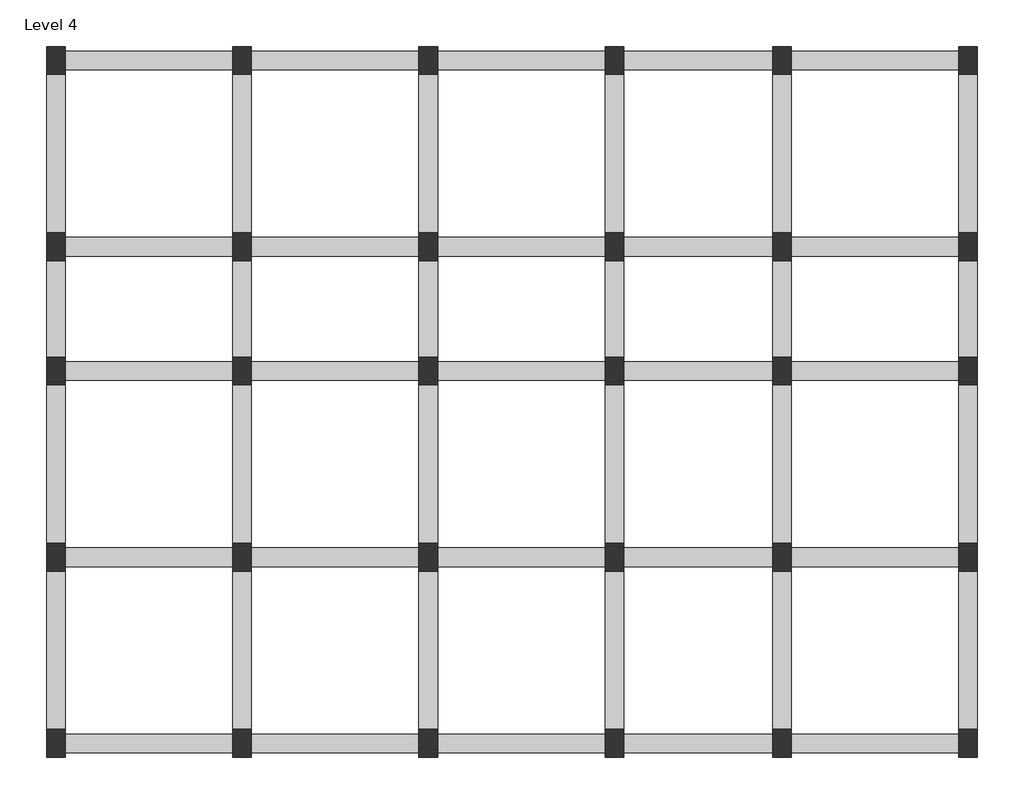
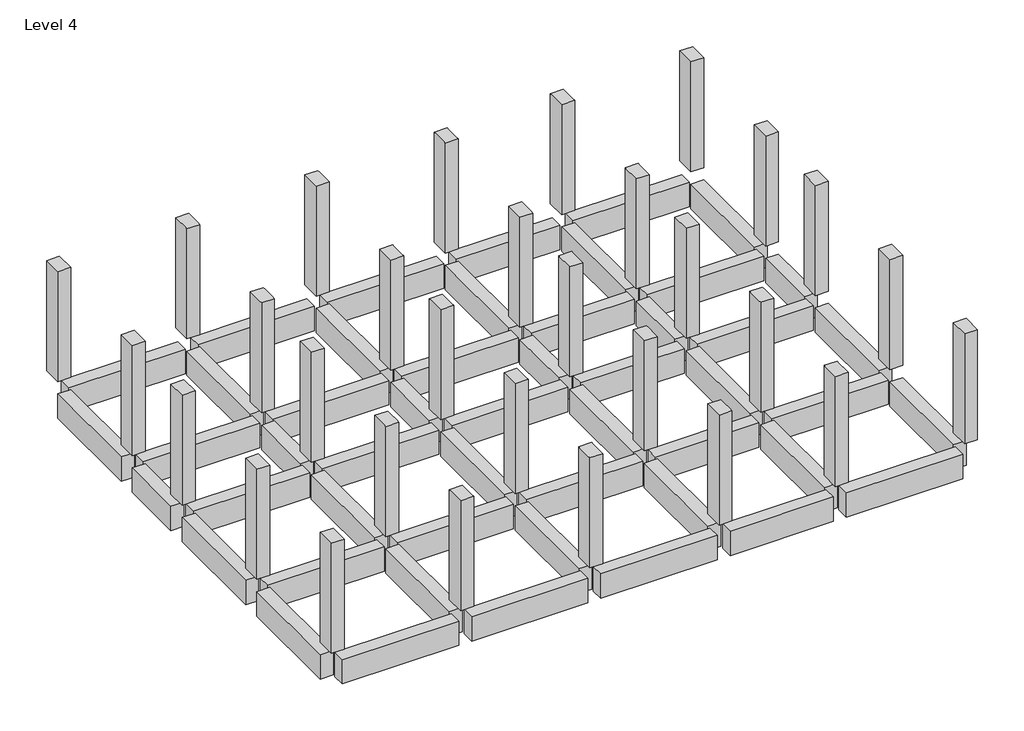
# One storey: 30 columns, 11 beams.
"""IFC4 building model written with IfcOpenShell, lengths in millimetres."""

from ifc_helpers import new_model, si_unit, frame, origin, place, context, project, spatial, polyline, outline, extrude, faceted_brep, element, save

model = new_model("IFC4")

# Units and contexts
model_context = context("Model", 3, world=origin())
ifc_project = project(units=[si_unit("LENGTHUNIT", "METRE", prefix="MILLI")], contexts=[model_context])

# Site, building, storey
site = spatial("IfcSite", under=ifc_project)
building = spatial("IfcBuilding", under=site)
storey = spatial("IfcBuildingStorey", under=building, Name="Level 4", Elevation=9144.0)

# Beams
placement = place(None, origin())
element("IfcBeam", 1, ObjectType="Concrete-Rectangular Beam : 12 x 24", at=placement, inside=storey, context=model_context, shape_type="SweptSolid", body=[
    extrude(outline(polyline([(2607.7603583, 7596.6647757), (2607.7603583, 7291.8647757), (-135.4396417, 7291.8647757), (-135.4396417, 7596.6647757), (2607.7603583, 7596.6647757)])), frame((0.0, 0.0, 8229.6), z_axis=(0.0, 0.0, 1.0), x_axis=(1.0, 0.0, 0.0)), (0.0, 0.0, 1.0), 609.6),
    extrude(outline(polyline([(-12022.6396417, 7291.8647757), (-12022.6396417, 7596.6647757), (-9279.4396417, 7596.6647757), (-9279.4396417, 7291.8647757), (-12022.6396417, 7291.8647757)])), frame((0.0, 0.0, 8229.6), z_axis=(0.0, 0.0, 1.0), x_axis=(1.0, 0.0, 0.0)), (0.0, 0.0, 1.0), 609.6),
    extrude(outline(polyline([(-8974.6396417, 7291.8647757), (-8974.6396417, 7596.6647757), (-6231.4396417, 7596.6647757), (-6231.4396417, 7291.8647757), (-8974.6396417, 7291.8647757)])), frame((0.0, 0.0, 8229.6), z_axis=(0.0, 0.0, 1.0), x_axis=(1.0, 0.0, 0.0)), (0.0, 0.0, 1.0), 609.6),
    extrude(outline(polyline([(-5926.6396417, 7291.8647757), (-5926.6396417, 7596.6647757), (-3183.4396417, 7596.6647757), (-3183.4396417, 7291.8647757), (-5926.6396417, 7291.8647757)])), frame((0.0, 0.0, 8229.6), z_axis=(0.0, 0.0, 1.0), x_axis=(1.0, 0.0, 0.0)), (0.0, 0.0, 1.0), 609.6),
    extrude(outline(polyline([(-2878.6396417, 7291.8647757), (-2878.6396417, 7596.6647757), (-440.2396417, 7596.6647757), (-440.2396417, 7291.8647757), (-2878.6396417, 7291.8647757)])), frame((0.0, 0.0, 8229.6), z_axis=(0.0, 0.0, 1.0), x_axis=(1.0, 0.0, 0.0)), (0.0, 0.0, 1.0), 609.6),
])
element("IfcBeam", 2, ObjectType="Concrete-Rectangular Beam : 12 x 24", at=placement, inside=storey, context=model_context, shape_type="SweptSolid", body=[
    extrude(outline(polyline([(2607.7603583, 10644.6647757), (2607.7603583, 10339.8647757), (-135.4396417, 10339.8647757), (-135.4396417, 10644.6647757), (2607.7603583, 10644.6647757)])), frame((0.0, 0.0, 8229.6), z_axis=(0.0, 0.0, 1.0), x_axis=(1.0, 0.0, 0.0)), (0.0, 0.0, 1.0), 609.6),
    extrude(outline(polyline([(-12022.6396417, 10339.8647757), (-12022.6396417, 10644.6647757), (-9279.4396417, 10644.6647757), (-9279.4396417, 10339.8647757), (-12022.6396417, 10339.8647757)])), frame((0.0, 0.0, 8229.6), z_axis=(0.0, 0.0, 1.0), x_axis=(1.0, 0.0, 0.0)), (0.0, 0.0, 1.0), 609.6),
    extrude(outline(polyline([(-8974.6396417, 10339.8647757), (-8974.6396417, 10644.6647757), (-6231.4396417, 10644.6647757), (-6231.4396417, 10339.8647757), (-8974.6396417, 10339.8647757)])), frame((0.0, 0.0, 8229.6), z_axis=(0.0, 0.0, 1.0), x_axis=(1.0, 0.0, 0.0)), (0.0, 0.0, 1.0), 609.6),
    extrude(outline(polyline([(-5926.6396417, 10339.8647757), (-5926.6396417, 10644.6647757), (-3183.4396417, 10644.6647757), (-3183.4396417, 10339.8647757), (-5926.6396417, 10339.8647757)])), frame((0.0, 0.0, 8229.6), z_axis=(0.0, 0.0, 1.0), x_axis=(1.0, 0.0, 0.0)), (0.0, 0.0, 1.0), 609.6),
    extrude(outline(polyline([(-2878.6396417, 10339.8647757), (-2878.6396417, 10644.6647757), (-440.2396417, 10644.6647757), (-440.2396417, 10339.8647757), (-2878.6396417, 10339.8647757)])), frame((0.0, 0.0, 8229.6), z_axis=(0.0, 0.0, 1.0), x_axis=(1.0, 0.0, 0.0)), (0.0, 0.0, 1.0), 609.6),
])
element("IfcBeam", 3, ObjectType="Concrete-Rectangular Beam : 12 x 24", at=placement, inside=storey, context=model_context, shape_type="SweptSolid", body=[
    extrude(outline(polyline([(2607.7603583, 13692.6647757), (2607.7603583, 13387.8647757), (-135.4396417, 13387.8647757), (-135.4396417, 13692.6647757), (2607.7603583, 13692.6647757)])), frame((0.0, 0.0, 8229.6), z_axis=(0.0, 0.0, 1.0), x_axis=(1.0, 0.0, 0.0)), (0.0, 0.0, 1.0), 609.6),
    extrude(outline(polyline([(-12022.6396417, 13387.8647757), (-12022.6396417, 13692.6647757), (-9279.4396417, 13692.6647757), (-9279.4396417, 13387.8647757), (-12022.6396417, 13387.8647757)])), frame((0.0, 0.0, 8229.6), z_axis=(0.0, 0.0, 1.0), x_axis=(1.0, 0.0, 0.0)), (0.0, 0.0, 1.0), 609.6),
    extrude(outline(polyline([(-8974.6396417, 13387.8647757), (-8974.6396417, 13692.6647757), (-6231.4396417, 13692.6647757), (-6231.4396417, 13387.8647757), (-8974.6396417, 13387.8647757)])), frame((0.0, 0.0, 8229.6), z_axis=(0.0, 0.0, 1.0), x_axis=(1.0, 0.0, 0.0)), (0.0, 0.0, 1.0), 609.6),
    extrude(outline(polyline([(-5926.6396417, 13387.8647757), (-5926.6396417, 13692.6647757), (-3183.4396417, 13692.6647757), (-3183.4396417, 13387.8647757), (-5926.6396417, 13387.8647757)])), frame((0.0, 0.0, 8229.6), z_axis=(0.0, 0.0, 1.0), x_axis=(1.0, 0.0, 0.0)), (0.0, 0.0, 1.0), 609.6),
    extrude(outline(polyline([(-2878.6396417, 13387.8647757), (-2878.6396417, 13692.6647757), (-440.2396417, 13692.6647757), (-440.2396417, 13387.8647757), (-2878.6396417, 13387.8647757)])), frame((0.0, 0.0, 8229.6), z_axis=(0.0, 0.0, 1.0), x_axis=(1.0, 0.0, 0.0)), (0.0, 0.0, 1.0), 609.6),
])
element("IfcBeam", 4, ObjectType="Concrete-Rectangular Beam : 12 x 24", at=placement, inside=storey, context=model_context, shape_type="SweptSolid", body=[
    extrude(outline(polyline([(2607.7603583, 15727.9119241), (2607.7603583, 15423.1119241), (-135.4396417, 15423.1119241), (-135.4396417, 15727.9119241), (2607.7603583, 15727.9119241)])), frame((0.0, 0.0, 8229.6), z_axis=(0.0, 0.0, 1.0), x_axis=(1.0, 0.0, 0.0)), (0.0, 0.0, 1.0), 609.6),
    extrude(outline(polyline([(-12022.6396417, 15423.1119241), (-12022.6396417, 15727.9119241), (-9279.4396417, 15727.9119241), (-9279.4396417, 15423.1119241), (-12022.6396417, 15423.1119241)])), frame((0.0, 0.0, 8229.6), z_axis=(0.0, 0.0, 1.0), x_axis=(1.0, 0.0, 0.0)), (0.0, 0.0, 1.0), 609.6),
    extrude(outline(polyline([(-8974.6396417, 15423.1119241), (-8974.6396417, 15727.9119241), (-6231.4396417, 15727.9119241), (-6231.4396417, 15423.1119241), (-8974.6396417, 15423.1119241)])), frame((0.0, 0.0, 8229.6), z_axis=(0.0, 0.0, 1.0), x_axis=(1.0, 0.0, 0.0)), (0.0, 0.0, 1.0), 609.6),
    extrude(outline(polyline([(-5926.6396417, 15423.1119241), (-5926.6396417, 15727.9119241), (-3183.4396417, 15727.9119241), (-3183.4396417, 15423.1119241), (-5926.6396417, 15423.1119241)])), frame((0.0, 0.0, 8229.6), z_axis=(0.0, 0.0, 1.0), x_axis=(1.0, 0.0, 0.0)), (0.0, 0.0, 1.0), 609.6),
    extrude(outline(polyline([(-2878.6396417, 15423.1119241), (-2878.6396417, 15727.9119241), (-440.2396417, 15727.9119241), (-440.2396417, 15423.1119241), (-2878.6396417, 15423.1119241)])), frame((0.0, 0.0, 8229.6), z_axis=(0.0, 0.0, 1.0), x_axis=(1.0, 0.0, 0.0)), (0.0, 0.0, 1.0), 609.6),
])
element("IfcBeam", 5, ObjectType="Concrete-Rectangular Beam : 12 x 24", at=placement, inside=storey, context=model_context, shape_type="SweptSolid", body=[
    extrude(outline(polyline([(2607.7603583, 18775.9119241), (2607.7603583, 18471.1119241), (-135.4396417, 18471.1119241), (-135.4396417, 18775.9119241), (2607.7603583, 18775.9119241)])), frame((0.0, 0.0, 8229.6), z_axis=(0.0, 0.0, 1.0), x_axis=(1.0, 0.0, 0.0)), (0.0, 0.0, 1.0), 609.6),
    extrude(outline(polyline([(-12022.6396417, 18471.1119241), (-12022.6396417, 18775.9119241), (-9279.4396417, 18775.9119241), (-9279.4396417, 18471.1119241), (-12022.6396417, 18471.1119241)])), frame((0.0, 0.0, 8229.6), z_axis=(0.0, 0.0, 1.0), x_axis=(1.0, 0.0, 0.0)), (0.0, 0.0, 1.0), 609.6),
    extrude(outline(polyline([(-8974.6396417, 18471.1119241), (-8974.6396417, 18775.9119241), (-6231.4396417, 18775.9119241), (-6231.4396417, 18471.1119241), (-8974.6396417, 18471.1119241)])), frame((0.0, 0.0, 8229.6), z_axis=(0.0, 0.0, 1.0), x_axis=(1.0, 0.0, 0.0)), (0.0, 0.0, 1.0), 609.6),
    extrude(outline(polyline([(-5926.6396417, 18471.1119241), (-5926.6396417, 18775.9119241), (-3183.4396417, 18775.9119241), (-3183.4396417, 18471.1119241), (-5926.6396417, 18471.1119241)])), frame((0.0, 0.0, 8229.6), z_axis=(0.0, 0.0, 1.0), x_axis=(1.0, 0.0, 0.0)), (0.0, 0.0, 1.0), 609.6),
    extrude(outline(polyline([(-2878.6396417, 18471.1119241), (-2878.6396417, 18775.9119241), (-440.2396417, 18775.9119241), (-440.2396417, 18471.1119241), (-2878.6396417, 18471.1119241)])), frame((0.0, 0.0, 8229.6), z_axis=(0.0, 0.0, 1.0), x_axis=(1.0, 0.0, 0.0)), (0.0, 0.0, 1.0), 609.6),
])
element("IfcBeam", 6, ObjectType="Concrete-Rectangular Beam : 12 x 24", at=placement, inside=storey, context=model_context, shape_type="SweptSolid", body=[
    extrude(outline(polyline([(-12022.6396417, 7672.8647757), (-12327.4396417, 7672.8647757), (-12327.4396417, 10263.6647757), (-12022.6396417, 10263.6647757), (-12022.6396417, 7672.8647757)])), frame((0.0, 0.0, 8229.6), z_axis=(0.0, 0.0, 1.0), x_axis=(1.0, 0.0, 0.0)), (0.0, 0.0, 1.0), 609.6),
    extrude(outline(polyline([(-12327.4396417, 18394.9119241), (-12022.6396417, 18394.9119241), (-12022.6396417, 15804.1119241), (-12327.4396417, 15804.1119241), (-12327.4396417, 18394.9119241)])), frame((0.0, 0.0, 8229.6), z_axis=(0.0, 0.0, 1.0), x_axis=(1.0, 0.0, 0.0)), (0.0, 0.0, 1.0), 609.6),
    extrude(outline(polyline([(-12022.6396417, 10720.8647757), (-12327.4396417, 10720.8647757), (-12327.4396417, 13311.6647757), (-12022.6396417, 13311.6647757), (-12022.6396417, 10720.8647757)])), frame((0.0, 0.0, 8229.6), z_axis=(0.0, 0.0, 1.0), x_axis=(1.0, 0.0, 0.0)), (0.0, 0.0, 1.0), 609.6),
    extrude(outline(polyline([(-12022.6396417, 13768.8647757), (-12327.4396417, 13768.8647757), (-12327.4396417, 15346.9119241), (-12022.6396417, 15346.9119241), (-12022.6396417, 13768.8647757)])), frame((0.0, 0.0, 8229.6), z_axis=(0.0, 0.0, 1.0), x_axis=(1.0, 0.0, 0.0)), (0.0, 0.0, 1.0), 609.6),
])
element("IfcBeam", 7, ObjectType="Concrete-Rectangular Beam : 12 x 24", at=placement, inside=storey, context=model_context, shape_type="SweptSolid", body=[
    extrude(outline(polyline([(-8974.6396417, 7672.8647757), (-9279.4396417, 7672.8647757), (-9279.4396417, 10263.6647757), (-8974.6396417, 10263.6647757), (-8974.6396417, 7672.8647757)])), frame((0.0, 0.0, 8229.6), z_axis=(0.0, 0.0, 1.0), x_axis=(1.0, 0.0, 0.0)), (0.0, 0.0, 1.0), 609.6),
    extrude(outline(polyline([(-9279.4396417, 18394.9119241), (-8974.6396417, 18394.9119241), (-8974.6396417, 15804.1119241), (-9279.4396417, 15804.1119241), (-9279.4396417, 18394.9119241)])), frame((0.0, 0.0, 8229.6), z_axis=(0.0, 0.0, 1.0), x_axis=(1.0, 0.0, 0.0)), (0.0, 0.0, 1.0), 609.6),
    extrude(outline(polyline([(-8974.6396417, 10720.8647757), (-9279.4396417, 10720.8647757), (-9279.4396417, 13311.6647757), (-8974.6396417, 13311.6647757), (-8974.6396417, 10720.8647757)])), frame((0.0, 0.0, 8229.6), z_axis=(0.0, 0.0, 1.0), x_axis=(1.0, 0.0, 0.0)), (0.0, 0.0, 1.0), 609.6),
    extrude(outline(polyline([(-8974.6396417, 13768.8647757), (-9279.4396417, 13768.8647757), (-9279.4396417, 15346.9119241), (-8974.6396417, 15346.9119241), (-8974.6396417, 13768.8647757)])), frame((0.0, 0.0, 8229.6), z_axis=(0.0, 0.0, 1.0), x_axis=(1.0, 0.0, 0.0)), (0.0, 0.0, 1.0), 609.6),
])
element("IfcBeam", 8, ObjectType="Concrete-Rectangular Beam : 12 x 24", at=placement, inside=storey, context=model_context, shape_type="SweptSolid", body=[
    extrude(outline(polyline([(-5926.6396417, 7672.8647757), (-6231.4396417, 7672.8647757), (-6231.4396417, 10263.6647757), (-5926.6396417, 10263.6647757), (-5926.6396417, 7672.8647757)])), frame((0.0, 0.0, 8229.6), z_axis=(0.0, 0.0, 1.0), x_axis=(1.0, 0.0, 0.0)), (0.0, 0.0, 1.0), 609.6),
    extrude(outline(polyline([(-6231.4396417, 18394.9119241), (-5926.6396417, 18394.9119241), (-5926.6396417, 15804.1119241), (-6231.4396417, 15804.1119241), (-6231.4396417, 18394.9119241)])), frame((0.0, 0.0, 8229.6), z_axis=(0.0, 0.0, 1.0), x_axis=(1.0, 0.0, 0.0)), (0.0, 0.0, 1.0), 609.6),
    extrude(outline(polyline([(-5926.6396417, 10720.8647757), (-6231.4396417, 10720.8647757), (-6231.4396417, 13311.6647757), (-5926.6396417, 13311.6647757), (-5926.6396417, 10720.8647757)])), frame((0.0, 0.0, 8229.6), z_axis=(0.0, 0.0, 1.0), x_axis=(1.0, 0.0, 0.0)), (0.0, 0.0, 1.0), 609.6),
    extrude(outline(polyline([(-5926.6396417, 13768.8647757), (-6231.4396417, 13768.8647757), (-6231.4396417, 15346.9119241), (-5926.6396417, 15346.9119241), (-5926.6396417, 13768.8647757)])), frame((0.0, 0.0, 8229.6), z_axis=(0.0, 0.0, 1.0), x_axis=(1.0, 0.0, 0.0)), (0.0, 0.0, 1.0), 609.6),
])
element("IfcBeam", 9, ObjectType="Concrete-Rectangular Beam : 12 x 24", at=placement, inside=storey, context=model_context, shape_type="SweptSolid", body=[
    extrude(outline(polyline([(-2878.6396417, 7672.8647757), (-3183.4396417, 7672.8647757), (-3183.4396417, 10263.6647757), (-2878.6396417, 10263.6647757), (-2878.6396417, 7672.8647757)])), frame((0.0, 0.0, 8229.6), z_axis=(0.0, 0.0, 1.0), x_axis=(1.0, 0.0, 0.0)), (0.0, 0.0, 1.0), 609.6),
    extrude(outline(polyline([(-3183.4396417, 18394.9119241), (-2878.6396417, 18394.9119241), (-2878.6396417, 15804.1119241), (-3183.4396417, 15804.1119241), (-3183.4396417, 18394.9119241)])), frame((0.0, 0.0, 8229.6), z_axis=(0.0, 0.0, 1.0), x_axis=(1.0, 0.0, 0.0)), (0.0, 0.0, 1.0), 609.6),
    extrude(outline(polyline([(-2878.6396417, 10720.8647757), (-3183.4396417, 10720.8647757), (-3183.4396417, 13311.6647757), (-2878.6396417, 13311.6647757), (-2878.6396417, 10720.8647757)])), frame((0.0, 0.0, 8229.6), z_axis=(0.0, 0.0, 1.0), x_axis=(1.0, 0.0, 0.0)), (0.0, 0.0, 1.0), 609.6),
    extrude(outline(polyline([(-2878.6396417, 13768.8647757), (-3183.4396417, 13768.8647757), (-3183.4396417, 15346.9119241), (-2878.6396417, 15346.9119241), (-2878.6396417, 13768.8647757)])), frame((0.0, 0.0, 8229.6), z_axis=(0.0, 0.0, 1.0), x_axis=(1.0, 0.0, 0.0)), (0.0, 0.0, 1.0), 609.6),
])
element("IfcBeam", 10, ObjectType="Concrete-Rectangular Beam : 12 x 24", at=placement, inside=storey, context=model_context, shape_type="SweptSolid", body=[
    extrude(outline(polyline([(-135.4396417, 7672.8647757), (-440.2396417, 7672.8647757), (-440.2396417, 10263.6647757), (-135.4396417, 10263.6647757), (-135.4396417, 7672.8647757)])), frame((0.0, 0.0, 8229.6), z_axis=(0.0, 0.0, 1.0), x_axis=(1.0, 0.0, 0.0)), (0.0, 0.0, 1.0), 609.6),
    extrude(outline(polyline([(-440.2396417, 18394.9119241), (-135.4396417, 18394.9119241), (-135.4396417, 15804.1119241), (-440.2396417, 15804.1119241), (-440.2396417, 18394.9119241)])), frame((0.0, 0.0, 8229.6), z_axis=(0.0, 0.0, 1.0), x_axis=(1.0, 0.0, 0.0)), (0.0, 0.0, 1.0), 609.6),
    extrude(outline(polyline([(-135.4396417, 10720.8647757), (-440.2396417, 10720.8647757), (-440.2396417, 13311.6647757), (-135.4396417, 13311.6647757), (-135.4396417, 10720.8647757)])), frame((0.0, 0.0, 8229.6), z_axis=(0.0, 0.0, 1.0), x_axis=(1.0, 0.0, 0.0)), (0.0, 0.0, 1.0), 609.6),
    extrude(outline(polyline([(-135.4396417, 13768.8647757), (-440.2396417, 13768.8647757), (-440.2396417, 15346.9119241), (-135.4396417, 15346.9119241), (-135.4396417, 13768.8647757)])), frame((0.0, 0.0, 8229.6), z_axis=(0.0, 0.0, 1.0), x_axis=(1.0, 0.0, 0.0)), (0.0, 0.0, 1.0), 609.6),
])
element("IfcBeam", 11, ObjectType="Concrete-Rectangular Beam : 12 x 24", at=placement, inside=storey, context=model_context, shape_type="SweptSolid", body=[
    extrude(outline(polyline([(2912.5603583, 7672.8647757), (2607.7603583, 7672.8647757), (2607.7603583, 10263.6647757), (2912.5603583, 10263.6647757), (2912.5603583, 7672.8647757)])), frame((0.0, 0.0, 8229.6), z_axis=(0.0, 0.0, 1.0), x_axis=(1.0, 0.0, 0.0)), (0.0, 0.0, 1.0), 609.6),
    extrude(outline(polyline([(2607.7603583, 18394.9119241), (2912.5603583, 18394.9119241), (2912.5603583, 15804.1119241), (2607.7603583, 15804.1119241), (2607.7603583, 18394.9119241)])), frame((0.0, 0.0, 8229.6), z_axis=(0.0, 0.0, 1.0), x_axis=(1.0, 0.0, 0.0)), (0.0, 0.0, 1.0), 609.6),
    extrude(outline(polyline([(2912.5603583, 10720.8647757), (2607.7603583, 10720.8647757), (2607.7603583, 13311.6647757), (2912.5603583, 13311.6647757), (2912.5603583, 10720.8647757)])), frame((0.0, 0.0, 8229.6), z_axis=(0.0, 0.0, 1.0), x_axis=(1.0, 0.0, 0.0)), (0.0, 0.0, 1.0), 609.6),
    extrude(outline(polyline([(2912.5603583, 13768.8647757), (2607.7603583, 13768.8647757), (2607.7603583, 15346.9119241), (2912.5603583, 15346.9119241), (2912.5603583, 13768.8647757)])), frame((0.0, 0.0, 8229.6), z_axis=(0.0, 0.0, 1.0), x_axis=(1.0, 0.0, 0.0)), (0.0, 0.0, 1.0), 609.6),
])

# Columns
element("IfcColumn", 12, ObjectType="Concrete-Rectangular-Column : c1", at=placement, inside=storey, context=model_context, shape_type="SweptSolid", body=[
    extrude(outline(polyline([(-12327.4396417, 7215.6647757), (-12327.4396417, 7672.8647757), (-12022.6396417, 7672.8647757), (-12022.6396417, 7215.6647757), (-12327.4396417, 7215.6647757)])), frame((0.0, 0.0, 9144.0), z_axis=(0.0, 0.0, 1.0), x_axis=(1.0, 0.0, 0.0)), (0.0, 0.0, 1.0), 2743.2),
])
element("IfcColumn", 13, ObjectType="Concrete-Rectangular-Column : c1", at=placement, inside=storey, context=model_context, shape_type="Brep", body=[
    faceted_brep([(-9279.4396417, 7215.6647757, 9144.0), (-9279.4396417, 7672.8647757, 9144.0), (-8974.6396417, 7672.8647757, 9144.0), (-8974.6396417, 7215.6647757, 9144.0), (-9279.4396417, 7215.6647757, 11887.2), (-9279.4396417, 7291.8647757, 11887.2), (-9279.4396417, 7596.6647757, 11887.2), (-9279.4396417, 7672.8647757, 11887.2), (-8974.6396417, 7672.8647757, 11887.2), (-8974.6396417, 7596.6647757, 11887.2), (-8974.6396417, 7291.8647757, 11887.2), (-8974.6396417, 7215.6647757, 11887.2)], [[[0, 1, 2, 3]], [[4, 5, 6, 7, 1, 0]], [[7, 8, 2, 1]], [[8, 9, 10, 11, 3, 2]], [[11, 4, 0, 3]], [[4, 11, 10, 9, 8, 7, 6, 5]]]),
])
element("IfcColumn", 14, ObjectType="Concrete-Rectangular-Column : c1", at=placement, inside=storey, context=model_context, shape_type="Brep", body=[
    faceted_brep([(-6231.4396417, 7215.6647757, 9144.0), (-6231.4396417, 7672.8647757, 9144.0), (-5926.6396417, 7672.8647757, 9144.0), (-5926.6396417, 7215.6647757, 9144.0), (-6231.4396417, 7215.6647757, 11887.2), (-6231.4396417, 7291.8647757, 11887.2), (-6231.4396417, 7596.6647757, 11887.2), (-6231.4396417, 7672.8647757, 11887.2), (-5926.6396417, 7672.8647757, 11887.2), (-5926.6396417, 7596.6647757, 11887.2), (-5926.6396417, 7291.8647757, 11887.2), (-5926.6396417, 7215.6647757, 11887.2)], [[[0, 1, 2, 3]], [[4, 5, 6, 7, 1, 0]], [[7, 8, 2, 1]], [[8, 9, 10, 11, 3, 2]], [[11, 4, 0, 3]], [[4, 11, 10, 9, 8, 7, 6, 5]]]),
])
element("IfcColumn", 15, ObjectType="Concrete-Rectangular-Column : c1", at=placement, inside=storey, context=model_context, shape_type="Brep", body=[
    faceted_brep([(-3183.4396417, 7215.6647757, 9144.0), (-3183.4396417, 7672.8647757, 9144.0), (-2878.6396417, 7672.8647757, 9144.0), (-2878.6396417, 7215.6647757, 9144.0), (-3183.4396417, 7215.6647757, 11887.2), (-3183.4396417, 7291.8647757, 11887.2), (-3183.4396417, 7596.6647757, 11887.2), (-3183.4396417, 7672.8647757, 11887.2), (-2878.6396417, 7672.8647757, 11887.2), (-2878.6396417, 7596.6647757, 11887.2), (-2878.6396417, 7291.8647757, 11887.2), (-2878.6396417, 7215.6647757, 11887.2)], [[[0, 1, 2, 3]], [[4, 5, 6, 7, 1, 0]], [[7, 8, 2, 1]], [[8, 9, 10, 11, 3, 2]], [[11, 4, 0, 3]], [[4, 11, 10, 9, 8, 7, 6, 5]]]),
])
element("IfcColumn", 16, ObjectType="Concrete-Rectangular-Column : c1", at=placement, inside=storey, context=model_context, shape_type="Brep", body=[
    faceted_brep([(-440.2396417, 7215.6647757, 9144.0), (-440.2396417, 7672.8647757, 9144.0), (-135.4396417, 7672.8647757, 9144.0), (-135.4396417, 7215.6647757, 9144.0), (-440.2396417, 7215.6647757, 11887.2), (-440.2396417, 7291.8647757, 11887.2), (-440.2396417, 7596.6647757, 11887.2), (-440.2396417, 7672.8647757, 11887.2), (-135.4396417, 7672.8647757, 11887.2), (-135.4396417, 7596.6647757, 11887.2), (-135.4396417, 7291.8647757, 11887.2), (-135.4396417, 7215.6647757, 11887.2)], [[[0, 1, 2, 3]], [[4, 5, 6, 7, 1, 0]], [[7, 8, 2, 1]], [[8, 9, 10, 11, 3, 2]], [[11, 4, 0, 3]], [[4, 11, 10, 9, 8, 7, 6, 5]]]),
])
element("IfcColumn", 17, ObjectType="Concrete-Rectangular-Column : c1", at=placement, inside=storey, context=model_context, shape_type="SweptSolid", body=[
    extrude(outline(polyline([(2607.7603583, 7215.6647757), (2607.7603583, 7672.8647757), (2912.5603583, 7672.8647757), (2912.5603583, 7215.6647757), (2607.7603583, 7215.6647757)])), frame((0.0, 0.0, 9144.0), z_axis=(0.0, 0.0, 1.0), x_axis=(1.0, 0.0, 0.0)), (0.0, 0.0, 1.0), 2743.2),
])
element("IfcColumn", 18, ObjectType="Concrete-Rectangular-Column : c1", at=placement, inside=storey, context=model_context, shape_type="Brep", body=[
    faceted_brep([(-12327.4396417, 10263.6647757, 9144.0), (-12327.4396417, 10720.8647757, 9144.0), (-12022.6396417, 10720.8647757, 9144.0), (-12022.6396417, 10263.6647757, 9144.0), (-12327.4396417, 10263.6647757, 11887.2), (-12327.4396417, 10720.8647757, 11887.2), (-12327.4396417, 10720.8647757, 11277.6), (-12327.4396417, 10263.6647757, 11277.6), (-12022.6396417, 10720.8647757, 11887.2), (-12022.6396417, 10720.8647757, 11277.6), (-12022.6396417, 10263.6647757, 11887.2), (-12022.6396417, 10263.6647757, 11277.6)], [[[0, 1, 2, 3]], [[4, 5, 6, 1, 0, 7]], [[5, 8, 9, 2, 1, 6]], [[8, 10, 11, 3, 2, 9]], [[10, 4, 7, 0, 3, 11]], [[4, 10, 8, 5]]]),
])
element("IfcColumn", 19, ObjectType="Concrete-Rectangular-Column : c1", at=placement, inside=storey, context=model_context, shape_type="Brep", body=[
    faceted_brep([(-9279.4396417, 10263.6647757, 9144.0), (-9279.4396417, 10720.8647757, 9144.0), (-8974.6396417, 10720.8647757, 9144.0), (-8974.6396417, 10263.6647757, 9144.0), (-9279.4396417, 10263.6647757, 11887.2), (-9279.4396417, 10339.8647757, 11887.2), (-9279.4396417, 10644.6647757, 11887.2), (-9279.4396417, 10720.8647757, 11887.2), (-9279.4396417, 10720.8647757, 11277.6), (-9279.4396417, 10263.6647757, 11277.6), (-8974.6396417, 10720.8647757, 11887.2), (-8974.6396417, 10720.8647757, 11277.6), (-8974.6396417, 10644.6647757, 11887.2), (-8974.6396417, 10339.8647757, 11887.2), (-8974.6396417, 10263.6647757, 11887.2), (-8974.6396417, 10263.6647757, 11277.6)], [[[0, 1, 2, 3]], [[4, 5, 6, 7, 8, 1, 0, 9]], [[7, 10, 11, 2, 1, 8]], [[10, 12, 13, 14, 15, 3, 2, 11]], [[14, 4, 9, 0, 3, 15]], [[4, 14, 13, 12, 10, 7, 6, 5]]]),
])
element("IfcColumn", 20, ObjectType="Concrete-Rectangular-Column : c1", at=placement, inside=storey, context=model_context, shape_type="Brep", body=[
    faceted_brep([(-6231.4396417, 10263.6647757, 9144.0), (-6231.4396417, 10720.8647757, 9144.0), (-5926.6396417, 10720.8647757, 9144.0), (-5926.6396417, 10263.6647757, 9144.0), (-6231.4396417, 10263.6647757, 11887.2), (-6231.4396417, 10339.8647757, 11887.2), (-6231.4396417, 10644.6647757, 11887.2), (-6231.4396417, 10720.8647757, 11887.2), (-6231.4396417, 10720.8647757, 11277.6), (-6231.4396417, 10263.6647757, 11277.6), (-5926.6396417, 10720.8647757, 11887.2), (-5926.6396417, 10720.8647757, 11277.6), (-5926.6396417, 10644.6647757, 11887.2), (-5926.6396417, 10339.8647757, 11887.2), (-5926.6396417, 10263.6647757, 11887.2), (-5926.6396417, 10263.6647757, 11277.6)], [[[0, 1, 2, 3]], [[4, 5, 6, 7, 8, 1, 0, 9]], [[7, 10, 11, 2, 1, 8]], [[10, 12, 13, 14, 15, 3, 2, 11]], [[14, 4, 9, 0, 3, 15]], [[4, 14, 13, 12, 10, 7, 6, 5]]]),
])
element("IfcColumn", 21, ObjectType="Concrete-Rectangular-Column : c1", at=placement, inside=storey, context=model_context, shape_type="Brep", body=[
    faceted_brep([(-3183.4396417, 10263.6647757, 9144.0), (-3183.4396417, 10720.8647757, 9144.0), (-2878.6396417, 10720.8647757, 9144.0), (-2878.6396417, 10263.6647757, 9144.0), (-3183.4396417, 10263.6647757, 11887.2), (-3183.4396417, 10339.8647757, 11887.2), (-3183.4396417, 10644.6647757, 11887.2), (-3183.4396417, 10720.8647757, 11887.2), (-3183.4396417, 10720.8647757, 11277.6), (-3183.4396417, 10263.6647757, 11277.6), (-2878.6396417, 10720.8647757, 11887.2), (-2878.6396417, 10720.8647757, 11277.6), (-2878.6396417, 10644.6647757, 11887.2), (-2878.6396417, 10339.8647757, 11887.2), (-2878.6396417, 10263.6647757, 11887.2), (-2878.6396417, 10263.6647757, 11277.6)], [[[0, 1, 2, 3]], [[4, 5, 6, 7, 8, 1, 0, 9]], [[7, 10, 11, 2, 1, 8]], [[10, 12, 13, 14, 15, 3, 2, 11]], [[14, 4, 9, 0, 3, 15]], [[4, 14, 13, 12, 10, 7, 6, 5]]]),
])
element("IfcColumn", 22, ObjectType="Concrete-Rectangular-Column : c1", at=placement, inside=storey, context=model_context, shape_type="Brep", body=[
    faceted_brep([(-440.2396417, 10263.6647757, 9144.0), (-440.2396417, 10720.8647757, 9144.0), (-135.4396417, 10720.8647757, 9144.0), (-135.4396417, 10263.6647757, 9144.0), (-440.2396417, 10263.6647757, 11887.2), (-440.2396417, 10339.8647757, 11887.2), (-440.2396417, 10644.6647757, 11887.2), (-440.2396417, 10720.8647757, 11887.2), (-440.2396417, 10720.8647757, 11277.6), (-440.2396417, 10263.6647757, 11277.6), (-135.4396417, 10720.8647757, 11887.2), (-135.4396417, 10720.8647757, 11277.6), (-135.4396417, 10644.6647757, 11887.2), (-135.4396417, 10339.8647757, 11887.2), (-135.4396417, 10263.6647757, 11887.2), (-135.4396417, 10263.6647757, 11277.6)], [[[0, 1, 2, 3]], [[4, 5, 6, 7, 8, 1, 0, 9]], [[7, 10, 11, 2, 1, 8]], [[10, 12, 13, 14, 15, 3, 2, 11]], [[14, 4, 9, 0, 3, 15]], [[4, 14, 13, 12, 10, 7, 6, 5]]]),
])
element("IfcColumn", 23, ObjectType="Concrete-Rectangular-Column : c1", at=placement, inside=storey, context=model_context, shape_type="Brep", body=[
    faceted_brep([(2607.7603583, 10263.6647757, 9144.0), (2607.7603583, 10720.8647757, 9144.0), (2912.5603583, 10720.8647757, 9144.0), (2912.5603583, 10263.6647757, 9144.0), (2607.7603583, 10263.6647757, 11887.2), (2607.7603583, 10720.8647757, 11887.2), (2607.7603583, 10720.8647757, 11277.6), (2607.7603583, 10263.6647757, 11277.6), (2912.5603583, 10720.8647757, 11887.2), (2912.5603583, 10720.8647757, 11277.6), (2912.5603583, 10263.6647757, 11887.2), (2912.5603583, 10263.6647757, 11277.6)], [[[0, 1, 2, 3]], [[4, 5, 6, 1, 0, 7]], [[5, 8, 9, 2, 1, 6]], [[8, 10, 11, 3, 2, 9]], [[10, 4, 7, 0, 3, 11]], [[4, 10, 8, 5]]]),
])
element("IfcColumn", 24, ObjectType="Concrete-Rectangular-Column : c1", at=placement, inside=storey, context=model_context, shape_type="Brep", body=[
    faceted_brep([(-12327.4396417, 13311.6647757, 9144.0), (-12327.4396417, 13768.8647757, 9144.0), (-12022.6396417, 13768.8647757, 9144.0), (-12022.6396417, 13311.6647757, 9144.0), (-12327.4396417, 13311.6647757, 11887.2), (-12327.4396417, 13768.8647757, 11887.2), (-12327.4396417, 13768.8647757, 11277.6), (-12327.4396417, 13311.6647757, 11277.6), (-12022.6396417, 13768.8647757, 11887.2), (-12022.6396417, 13768.8647757, 11277.6), (-12022.6396417, 13311.6647757, 11887.2), (-12022.6396417, 13311.6647757, 11277.6)], [[[0, 1, 2, 3]], [[4, 5, 6, 1, 0, 7]], [[5, 8, 9, 2, 1, 6]], [[8, 10, 11, 3, 2, 9]], [[10, 4, 7, 0, 3, 11]], [[4, 10, 8, 5]]]),
])
element("IfcColumn", 25, ObjectType="Concrete-Rectangular-Column : c1", at=placement, inside=storey, context=model_context, shape_type="Brep", body=[
    faceted_brep([(-9279.4396417, 13311.6647757, 9144.0), (-9279.4396417, 13768.8647757, 9144.0), (-8974.6396417, 13768.8647757, 9144.0), (-8974.6396417, 13311.6647757, 9144.0), (-9279.4396417, 13311.6647757, 11887.2), (-9279.4396417, 13387.8647757, 11887.2), (-9279.4396417, 13692.6647757, 11887.2), (-9279.4396417, 13768.8647757, 11887.2), (-9279.4396417, 13768.8647757, 11277.6), (-9279.4396417, 13311.6647757, 11277.6), (-8974.6396417, 13768.8647757, 11887.2), (-8974.6396417, 13768.8647757, 11277.6), (-8974.6396417, 13692.6647757, 11887.2), (-8974.6396417, 13387.8647757, 11887.2), (-8974.6396417, 13311.6647757, 11887.2), (-8974.6396417, 13311.6647757, 11277.6)], [[[0, 1, 2, 3]], [[4, 5, 6, 7, 8, 1, 0, 9]], [[7, 10, 11, 2, 1, 8]], [[10, 12, 13, 14, 15, 3, 2, 11]], [[14, 4, 9, 0, 3, 15]], [[4, 14, 13, 12, 10, 7, 6, 5]]]),
])
element("IfcColumn", 26, ObjectType="Concrete-Rectangular-Column : c1", at=placement, inside=storey, context=model_context, shape_type="Brep", body=[
    faceted_brep([(-6231.4396417, 13311.6647757, 9144.0), (-6231.4396417, 13768.8647757, 9144.0), (-5926.6396417, 13768.8647757, 9144.0), (-5926.6396417, 13311.6647757, 9144.0), (-6231.4396417, 13311.6647757, 11887.2), (-6231.4396417, 13387.8647757, 11887.2), (-6231.4396417, 13692.6647757, 11887.2), (-6231.4396417, 13768.8647757, 11887.2), (-6231.4396417, 13768.8647757, 11277.6), (-6231.4396417, 13311.6647757, 11277.6), (-5926.6396417, 13768.8647757, 11887.2), (-5926.6396417, 13768.8647757, 11277.6), (-5926.6396417, 13692.6647757, 11887.2), (-5926.6396417, 13387.8647757, 11887.2), (-5926.6396417, 13311.6647757, 11887.2), (-5926.6396417, 13311.6647757, 11277.6)], [[[0, 1, 2, 3]], [[4, 5, 6, 7, 8, 1, 0, 9]], [[7, 10, 11, 2, 1, 8]], [[10, 12, 13, 14, 15, 3, 2, 11]], [[14, 4, 9, 0, 3, 15]], [[4, 14, 13, 12, 10, 7, 6, 5]]]),
])
element("IfcColumn", 27, ObjectType="Concrete-Rectangular-Column : c1", at=placement, inside=storey, context=model_context, shape_type="Brep", body=[
    faceted_brep([(-3183.4396417, 13311.6647757, 9144.0), (-3183.4396417, 13768.8647757, 9144.0), (-2878.6396417, 13768.8647757, 9144.0), (-2878.6396417, 13311.6647757, 9144.0), (-3183.4396417, 13311.6647757, 11887.2), (-3183.4396417, 13387.8647757, 11887.2), (-3183.4396417, 13692.6647757, 11887.2), (-3183.4396417, 13768.8647757, 11887.2), (-3183.4396417, 13768.8647757, 11277.6), (-3183.4396417, 13311.6647757, 11277.6), (-2878.6396417, 13768.8647757, 11887.2), (-2878.6396417, 13768.8647757, 11277.6), (-2878.6396417, 13692.6647757, 11887.2), (-2878.6396417, 13387.8647757, 11887.2), (-2878.6396417, 13311.6647757, 11887.2), (-2878.6396417, 13311.6647757, 11277.6)], [[[0, 1, 2, 3]], [[4, 5, 6, 7, 8, 1, 0, 9]], [[7, 10, 11, 2, 1, 8]], [[10, 12, 13, 14, 15, 3, 2, 11]], [[14, 4, 9, 0, 3, 15]], [[4, 14, 13, 12, 10, 7, 6, 5]]]),
])
element("IfcColumn", 28, ObjectType="Concrete-Rectangular-Column : c1", at=placement, inside=storey, context=model_context, shape_type="Brep", body=[
    faceted_brep([(-440.2396417, 13311.6647757, 9144.0), (-440.2396417, 13768.8647757, 9144.0), (-135.4396417, 13768.8647757, 9144.0), (-135.4396417, 13311.6647757, 9144.0), (-440.2396417, 13311.6647757, 11887.2), (-440.2396417, 13387.8647757, 11887.2), (-440.2396417, 13692.6647757, 11887.2), (-440.2396417, 13768.8647757, 11887.2), (-440.2396417, 13768.8647757, 11277.6), (-440.2396417, 13311.6647757, 11277.6), (-135.4396417, 13768.8647757, 11887.2), (-135.4396417, 13768.8647757, 11277.6), (-135.4396417, 13692.6647757, 11887.2), (-135.4396417, 13387.8647757, 11887.2), (-135.4396417, 13311.6647757, 11887.2), (-135.4396417, 13311.6647757, 11277.6)], [[[0, 1, 2, 3]], [[4, 5, 6, 7, 8, 1, 0, 9]], [[7, 10, 11, 2, 1, 8]], [[10, 12, 13, 14, 15, 3, 2, 11]], [[14, 4, 9, 0, 3, 15]], [[4, 14, 13, 12, 10, 7, 6, 5]]]),
])
element("IfcColumn", 29, ObjectType="Concrete-Rectangular-Column : c1", at=placement, inside=storey, context=model_context, shape_type="Brep", body=[
    faceted_brep([(2607.7603583, 13311.6647757, 9144.0), (2607.7603583, 13768.8647757, 9144.0), (2912.5603583, 13768.8647757, 9144.0), (2912.5603583, 13311.6647757, 9144.0), (2607.7603583, 13311.6647757, 11887.2), (2607.7603583, 13768.8647757, 11887.2), (2607.7603583, 13768.8647757, 11277.6), (2607.7603583, 13311.6647757, 11277.6), (2912.5603583, 13768.8647757, 11887.2), (2912.5603583, 13768.8647757, 11277.6), (2912.5603583, 13311.6647757, 11887.2), (2912.5603583, 13311.6647757, 11277.6)], [[[0, 1, 2, 3]], [[4, 5, 6, 1, 0, 7]], [[5, 8, 9, 2, 1, 6]], [[8, 10, 11, 3, 2, 9]], [[10, 4, 7, 0, 3, 11]], [[4, 10, 8, 5]]]),
])
element("IfcColumn", 30, ObjectType="Concrete-Rectangular-Column : c1", at=placement, inside=storey, context=model_context, shape_type="Brep", body=[
    faceted_brep([(-12327.4396417, 15346.9119241, 9144.0), (-12327.4396417, 15804.1119241, 9144.0), (-12022.6396417, 15804.1119241, 9144.0), (-12022.6396417, 15346.9119241, 9144.0), (-12327.4396417, 15346.9119241, 11887.2), (-12327.4396417, 15804.1119241, 11887.2), (-12327.4396417, 15804.1119241, 11277.6), (-12327.4396417, 15346.9119241, 11277.6), (-12022.6396417, 15804.1119241, 11887.2), (-12022.6396417, 15804.1119241, 11277.6), (-12022.6396417, 15346.9119241, 11887.2), (-12022.6396417, 15346.9119241, 11277.6)], [[[0, 1, 2, 3]], [[4, 5, 6, 1, 0, 7]], [[5, 8, 9, 2, 1, 6]], [[8, 10, 11, 3, 2, 9]], [[10, 4, 7, 0, 3, 11]], [[4, 10, 8, 5]]]),
])
element("IfcColumn", 31, ObjectType="Concrete-Rectangular-Column : c1", at=placement, inside=storey, context=model_context, shape_type="Brep", body=[
    faceted_brep([(-9279.4396417, 15346.9119241, 9144.0), (-9279.4396417, 15804.1119241, 9144.0), (-8974.6396417, 15804.1119241, 9144.0), (-8974.6396417, 15346.9119241, 9144.0), (-9279.4396417, 15346.9119241, 11887.2), (-9279.4396417, 15423.1119241, 11887.2), (-9279.4396417, 15727.9119241, 11887.2), (-9279.4396417, 15804.1119241, 11887.2), (-9279.4396417, 15804.1119241, 11277.6), (-9279.4396417, 15346.9119241, 11277.6), (-8974.6396417, 15804.1119241, 11887.2), (-8974.6396417, 15804.1119241, 11277.6), (-8974.6396417, 15727.9119241, 11887.2), (-8974.6396417, 15423.1119241, 11887.2), (-8974.6396417, 15346.9119241, 11887.2), (-8974.6396417, 15346.9119241, 11277.6)], [[[0, 1, 2, 3]], [[4, 5, 6, 7, 8, 1, 0, 9]], [[7, 10, 11, 2, 1, 8]], [[10, 12, 13, 14, 15, 3, 2, 11]], [[14, 4, 9, 0, 3, 15]], [[4, 14, 13, 12, 10, 7, 6, 5]]]),
])
element("IfcColumn", 32, ObjectType="Concrete-Rectangular-Column : c1", at=placement, inside=storey, context=model_context, shape_type="Brep", body=[
    faceted_brep([(-6231.4396417, 15346.9119241, 9144.0), (-6231.4396417, 15804.1119241, 9144.0), (-5926.6396417, 15804.1119241, 9144.0), (-5926.6396417, 15346.9119241, 9144.0), (-6231.4396417, 15346.9119241, 11887.2), (-6231.4396417, 15423.1119241, 11887.2), (-6231.4396417, 15727.9119241, 11887.2), (-6231.4396417, 15804.1119241, 11887.2), (-6231.4396417, 15804.1119241, 11277.6), (-6231.4396417, 15346.9119241, 11277.6), (-5926.6396417, 15804.1119241, 11887.2), (-5926.6396417, 15804.1119241, 11277.6), (-5926.6396417, 15727.9119241, 11887.2), (-5926.6396417, 15423.1119241, 11887.2), (-5926.6396417, 15346.9119241, 11887.2), (-5926.6396417, 15346.9119241, 11277.6)], [[[0, 1, 2, 3]], [[4, 5, 6, 7, 8, 1, 0, 9]], [[7, 10, 11, 2, 1, 8]], [[10, 12, 13, 14, 15, 3, 2, 11]], [[14, 4, 9, 0, 3, 15]], [[4, 14, 13, 12, 10, 7, 6, 5]]]),
])
element("IfcColumn", 33, ObjectType="Concrete-Rectangular-Column : c1", at=placement, inside=storey, context=model_context, shape_type="Brep", body=[
    faceted_brep([(-3183.4396417, 15346.9119241, 9144.0), (-3183.4396417, 15804.1119241, 9144.0), (-2878.6396417, 15804.1119241, 9144.0), (-2878.6396417, 15346.9119241, 9144.0), (-3183.4396417, 15346.9119241, 11887.2), (-3183.4396417, 15423.1119241, 11887.2), (-3183.4396417, 15727.9119241, 11887.2), (-3183.4396417, 15804.1119241, 11887.2), (-3183.4396417, 15804.1119241, 11277.6), (-3183.4396417, 15346.9119241, 11277.6), (-2878.6396417, 15804.1119241, 11887.2), (-2878.6396417, 15804.1119241, 11277.6), (-2878.6396417, 15727.9119241, 11887.2), (-2878.6396417, 15423.1119241, 11887.2), (-2878.6396417, 15346.9119241, 11887.2), (-2878.6396417, 15346.9119241, 11277.6)], [[[0, 1, 2, 3]], [[4, 5, 6, 7, 8, 1, 0, 9]], [[7, 10, 11, 2, 1, 8]], [[10, 12, 13, 14, 15, 3, 2, 11]], [[14, 4, 9, 0, 3, 15]], [[4, 14, 13, 12, 10, 7, 6, 5]]]),
])
element("IfcColumn", 34, ObjectType="Concrete-Rectangular-Column : c1", at=placement, inside=storey, context=model_context, shape_type="Brep", body=[
    faceted_brep([(-440.2396417, 15346.9119241, 9144.0), (-440.2396417, 15804.1119241, 9144.0), (-135.4396417, 15804.1119241, 9144.0), (-135.4396417, 15346.9119241, 9144.0), (-440.2396417, 15346.9119241, 11887.2), (-440.2396417, 15423.1119241, 11887.2), (-440.2396417, 15727.9119241, 11887.2), (-440.2396417, 15804.1119241, 11887.2), (-440.2396417, 15804.1119241, 11277.6), (-440.2396417, 15346.9119241, 11277.6), (-135.4396417, 15804.1119241, 11887.2), (-135.4396417, 15804.1119241, 11277.6), (-135.4396417, 15727.9119241, 11887.2), (-135.4396417, 15423.1119241, 11887.2), (-135.4396417, 15346.9119241, 11887.2), (-135.4396417, 15346.9119241, 11277.6)], [[[0, 1, 2, 3]], [[4, 5, 6, 7, 8, 1, 0, 9]], [[7, 10, 11, 2, 1, 8]], [[10, 12, 13, 14, 15, 3, 2, 11]], [[14, 4, 9, 0, 3, 15]], [[4, 14, 13, 12, 10, 7, 6, 5]]]),
])
element("IfcColumn", 35, ObjectType="Concrete-Rectangular-Column : c1", at=placement, inside=storey, context=model_context, shape_type="Brep", body=[
    faceted_brep([(2607.7603583, 15346.9119241, 9144.0), (2607.7603583, 15804.1119241, 9144.0), (2912.5603583, 15804.1119241, 9144.0), (2912.5603583, 15346.9119241, 9144.0), (2607.7603583, 15346.9119241, 11887.2), (2607.7603583, 15804.1119241, 11887.2), (2607.7603583, 15804.1119241, 11277.6), (2607.7603583, 15346.9119241, 11277.6), (2912.5603583, 15804.1119241, 11887.2), (2912.5603583, 15804.1119241, 11277.6), (2912.5603583, 15346.9119241, 11887.2), (2912.5603583, 15346.9119241, 11277.6)], [[[0, 1, 2, 3]], [[4, 5, 6, 1, 0, 7]], [[5, 8, 9, 2, 1, 6]], [[8, 10, 11, 3, 2, 9]], [[10, 4, 7, 0, 3, 11]], [[4, 10, 8, 5]]]),
])
element("IfcColumn", 36, ObjectType="Concrete-Rectangular-Column : c1", at=placement, inside=storey, context=model_context, shape_type="SweptSolid", body=[
    extrude(outline(polyline([(-12327.4396417, 18394.9119241), (-12327.4396417, 18852.1119241), (-12022.6396417, 18852.1119241), (-12022.6396417, 18394.9119241), (-12327.4396417, 18394.9119241)])), frame((0.0, 0.0, 9144.0), z_axis=(0.0, 0.0, 1.0), x_axis=(1.0, 0.0, 0.0)), (0.0, 0.0, 1.0), 2743.2),
])
element("IfcColumn", 37, ObjectType="Concrete-Rectangular-Column : c1", at=placement, inside=storey, context=model_context, shape_type="Brep", body=[
    faceted_brep([(-9279.4396417, 18394.9119241, 9144.0), (-9279.4396417, 18852.1119241, 9144.0), (-8974.6396417, 18852.1119241, 9144.0), (-8974.6396417, 18394.9119241, 9144.0), (-9279.4396417, 18394.9119241, 11887.2), (-9279.4396417, 18471.1119241, 11887.2), (-9279.4396417, 18775.9119241, 11887.2), (-9279.4396417, 18852.1119241, 11887.2), (-8974.6396417, 18852.1119241, 11887.2), (-8974.6396417, 18775.9119241, 11887.2), (-8974.6396417, 18471.1119241, 11887.2), (-8974.6396417, 18394.9119241, 11887.2)], [[[0, 1, 2, 3]], [[4, 5, 6, 7, 1, 0]], [[7, 8, 2, 1]], [[8, 9, 10, 11, 3, 2]], [[11, 4, 0, 3]], [[4, 11, 10, 9, 8, 7, 6, 5]]]),
])
element("IfcColumn", 38, ObjectType="Concrete-Rectangular-Column : c1", at=placement, inside=storey, context=model_context, shape_type="Brep", body=[
    faceted_brep([(-6231.4396417, 18394.9119241, 9144.0), (-6231.4396417, 18852.1119241, 9144.0), (-5926.6396417, 18852.1119241, 9144.0), (-5926.6396417, 18394.9119241, 9144.0), (-6231.4396417, 18394.9119241, 11887.2), (-6231.4396417, 18471.1119241, 11887.2), (-6231.4396417, 18775.9119241, 11887.2), (-6231.4396417, 18852.1119241, 11887.2), (-5926.6396417, 18852.1119241, 11887.2), (-5926.6396417, 18775.9119241, 11887.2), (-5926.6396417, 18471.1119241, 11887.2), (-5926.6396417, 18394.9119241, 11887.2)], [[[0, 1, 2, 3]], [[4, 5, 6, 7, 1, 0]], [[7, 8, 2, 1]], [[8, 9, 10, 11, 3, 2]], [[11, 4, 0, 3]], [[4, 11, 10, 9, 8, 7, 6, 5]]]),
])
element("IfcColumn", 39, ObjectType="Concrete-Rectangular-Column : c1", at=placement, inside=storey, context=model_context, shape_type="Brep", body=[
    faceted_brep([(-3183.4396417, 18394.9119241, 9144.0), (-3183.4396417, 18852.1119241, 9144.0), (-2878.6396417, 18852.1119241, 9144.0), (-2878.6396417, 18394.9119241, 9144.0), (-3183.4396417, 18394.9119241, 11887.2), (-3183.4396417, 18471.1119241, 11887.2), (-3183.4396417, 18775.9119241, 11887.2), (-3183.4396417, 18852.1119241, 11887.2), (-2878.6396417, 18852.1119241, 11887.2), (-2878.6396417, 18775.9119241, 11887.2), (-2878.6396417, 18471.1119241, 11887.2), (-2878.6396417, 18394.9119241, 11887.2)], [[[0, 1, 2, 3]], [[4, 5, 6, 7, 1, 0]], [[7, 8, 2, 1]], [[8, 9, 10, 11, 3, 2]], [[11, 4, 0, 3]], [[4, 11, 10, 9, 8, 7, 6, 5]]]),
])
element("IfcColumn", 40, ObjectType="Concrete-Rectangular-Column : c1", at=placement, inside=storey, context=model_context, shape_type="Brep", body=[
    faceted_brep([(-440.2396417, 18394.9119241, 9144.0), (-440.2396417, 18852.1119241, 9144.0), (-135.4396417, 18852.1119241, 9144.0), (-135.4396417, 18394.9119241, 9144.0), (-440.2396417, 18394.9119241, 11887.2), (-440.2396417, 18471.1119241, 11887.2), (-440.2396417, 18775.9119241, 11887.2), (-440.2396417, 18852.1119241, 11887.2), (-135.4396417, 18852.1119241, 11887.2), (-135.4396417, 18775.9119241, 11887.2), (-135.4396417, 18471.1119241, 11887.2), (-135.4396417, 18394.9119241, 11887.2)], [[[0, 1, 2, 3]], [[4, 5, 6, 7, 1, 0]], [[7, 8, 2, 1]], [[8, 9, 10, 11, 3, 2]], [[11, 4, 0, 3]], [[4, 11, 10, 9, 8, 7, 6, 5]]]),
])
element("IfcColumn", 41, ObjectType="Concrete-Rectangular-Column : c1", at=placement, inside=storey, context=model_context, shape_type="SweptSolid", body=[
    extrude(outline(polyline([(2607.7603583, 18394.9119241), (2607.7603583, 18852.1119241), (2912.5603583, 18852.1119241), (2912.5603583, 18394.9119241), (2607.7603583, 18394.9119241)])), frame((0.0, 0.0, 9144.0), z_axis=(0.0, 0.0, 1.0), x_axis=(1.0, 0.0, 0.0)), (0.0, 0.0, 1.0), 2743.2),
])

save(model, "model.ifc")

# Revit data of these elements
# Type "Concrete-Rectangular Beam : 12 x 24"
#   Assembly Code = "B10"
#   Length [instance default] = 5' - 0"
#   b = 1' - 0"
#   h = 2' - 0"
#   Structural Material [instance default] = Concrete, Cast-in-Place gray
# Type "Concrete-Rectangular-Column : c1"
#   Assembly Code = "B10"
#   b = 1' - 0"
#   h = 1' - 6"
#   Structural Material [instance default] = Concrete, Cast-in-Place gray
# Elements 1, 2, 3, 4, 5, 6, 7, 8, 9, 10, 11 (IfcBeam, "Concrete-Rectangular Beam : 12 x 24")
#   Structural Material = Concrete, Cast-in-Place gray
#   Phase Created = New Construction
#   Materials on its faces: "Concrete, Cast-in-Place gray"
# Elements 12, 13, 14, 15, 16, 17, 18, 19, 20, 21, 22, 23, 24, 25, 26, 27, 28, 29, 30, 31, 32, 33, 34, 35, 36, 37, 38, 39, 40, 41 (IfcColumn, "Concrete-Rectangular-Column : c1")
#   Comments = ""
#   Structural Material = Concrete, Cast-in-Place gray
#   Phase Created = New Construction
#   Materials on its faces: "Concrete, Cast-in-Place gray"
# Materials
#   "Concrete, Cast-in-Place gray": class "Concrete", colour RGB 192 192 192, transparency 0, Description = "Cast-in-place concrete", Cost = 0
